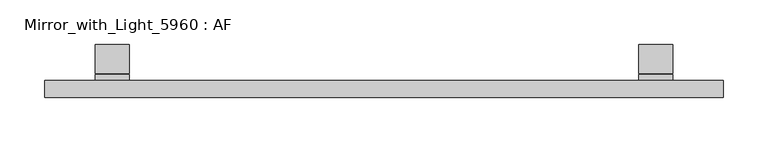
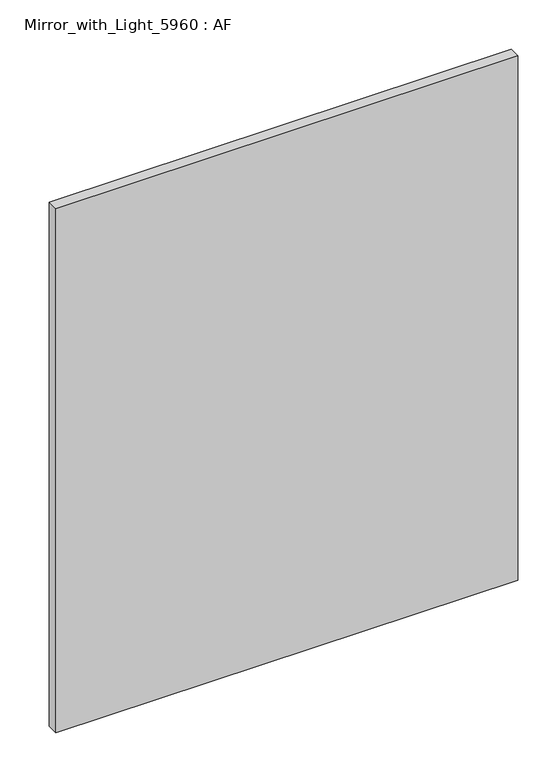
"""IFC4 building model written with IfcOpenShell, lengths in millimetres: flow terminal geometry, Mirror_with_Light_5960 : AF."""

from ifc_helpers import new_model, si_unit, frame, origin, place, context, project, spatial, polyline, outline, extrude, source, transform, mapped, element, save


def mirror_with_light_5960_af_41a2bd15(model_context):
    return source(origin(), model_context, "Body", "SweptSolid", [
        extrude(outline(polyline([(306.8695633, 88.9), (306.8695633, 95.25), (344.9695633, 95.25), (344.9695633, 88.9), (306.8695633, 88.9)])), frame((0.0, 0.0, 1371.6), z_axis=(0.0, 0.0, 1.0), x_axis=(1.0, 0.0, 0.0)), (0.0, 0.0, 1.0), 609.6),
        extrude(outline(polyline([(306.8695633, 96.8375), (306.8695633, 129.38125), (344.9695633, 129.38125), (344.9695633, 96.8375), (306.8695633, 96.8375)])), frame((0.0, 0.0, 1371.6), z_axis=(0.0, 0.0, 1.0), x_axis=(1.0, 0.0, 0.0)), (0.0, 0.0, 1.0), 609.6),
        extrude(outline(polyline([(-264.6304367, 88.9), (-302.7304367, 88.9), (-302.7304367, 95.25), (-264.6304367, 95.25), (-264.6304367, 88.9)])), frame((0.0, 0.0, 1371.6), z_axis=(0.0, 0.0, 1.0), x_axis=(1.0, 0.0, 0.0)), (0.0, 0.0, 1.0), 609.6),
        extrude(outline(polyline([(-264.6304367, 96.8375), (-302.7304367, 96.8375), (-302.7304367, 129.38125), (-264.6304367, 129.38125), (-264.6304367, 96.8375)])), frame((0.0, 0.0, 1371.6), z_axis=(0.0, 0.0, 1.0), x_axis=(1.0, 0.0, 0.0)), (0.0, 0.0, 1.0), 609.6),
        extrude(outline(polyline([(-359.8804367, 88.9), (402.1195633, 88.9), (402.1195633, 69.8833105), (-359.8804367, 69.8833105), (-359.8804367, 88.9)])), frame((0.0, 0.0, 1219.2), z_axis=(0.0, 0.0, 1.0), x_axis=(1.0, 0.0, 0.0)), (0.0, 0.0, 1.0), 914.4),
    ])


if __name__ == "__main__":
    model = new_model("IFC4")
    model_context = context("Model", 3, world=origin())
    ifc_project = project(units=[si_unit("LENGTHUNIT", "METRE", prefix="MILLI")], contexts=[model_context])
    site = spatial("IfcSite", under=ifc_project)
    building = spatial("IfcBuilding", under=site)
    placement = place(None, origin())
    mirror_with_light_5960_af_shape = mirror_with_light_5960_af_41a2bd15(model_context)
    element("IfcFlowTerminal", 1, ObjectType="Mirror_with_Light_5960 : AF", at=placement, inside=building, context=model_context, shape_type="MappedRepresentation", body=[
        mapped(mirror_with_light_5960_af_shape, transform((0.0, 0.0, 0.0), x_axis=(1.0, 0.0, 0.0), y_axis=(0.0, 1.0, 0.0), z_axis=(0.0, 0.0, 1.0))),
    ])
    save(model, "model.ifc")

# Revit data of these elements
# Type "Mirror_with_Light_5960 : AF"
#   Width [instance default] = 2' - 6"
#   Sill Hight [instance default] = 4' - 0"
#   Mirror Height = 3' - 0"
#   Depth [instance default] = 0' - 1"
#   Default Elevation = 0
#   Assembly Code = ""
# Element 1 (IfcFlowTerminal, "Mirror_with_Light_5960 : AF")
#   Materials on its faces: "Metal", "Glass 2", "Glass"
# Materials
#   "Metal": class "Generic", colour RGB 120 120 120, transparency 0, Cost = 0
#   "Glass 2": colour RGB 128 255 255, transparency 1
#   "Glass": class "Glass", colour RGB 0 128 192, transparency 0.9, Description = "Soda Lime Glass", Cost = 0
